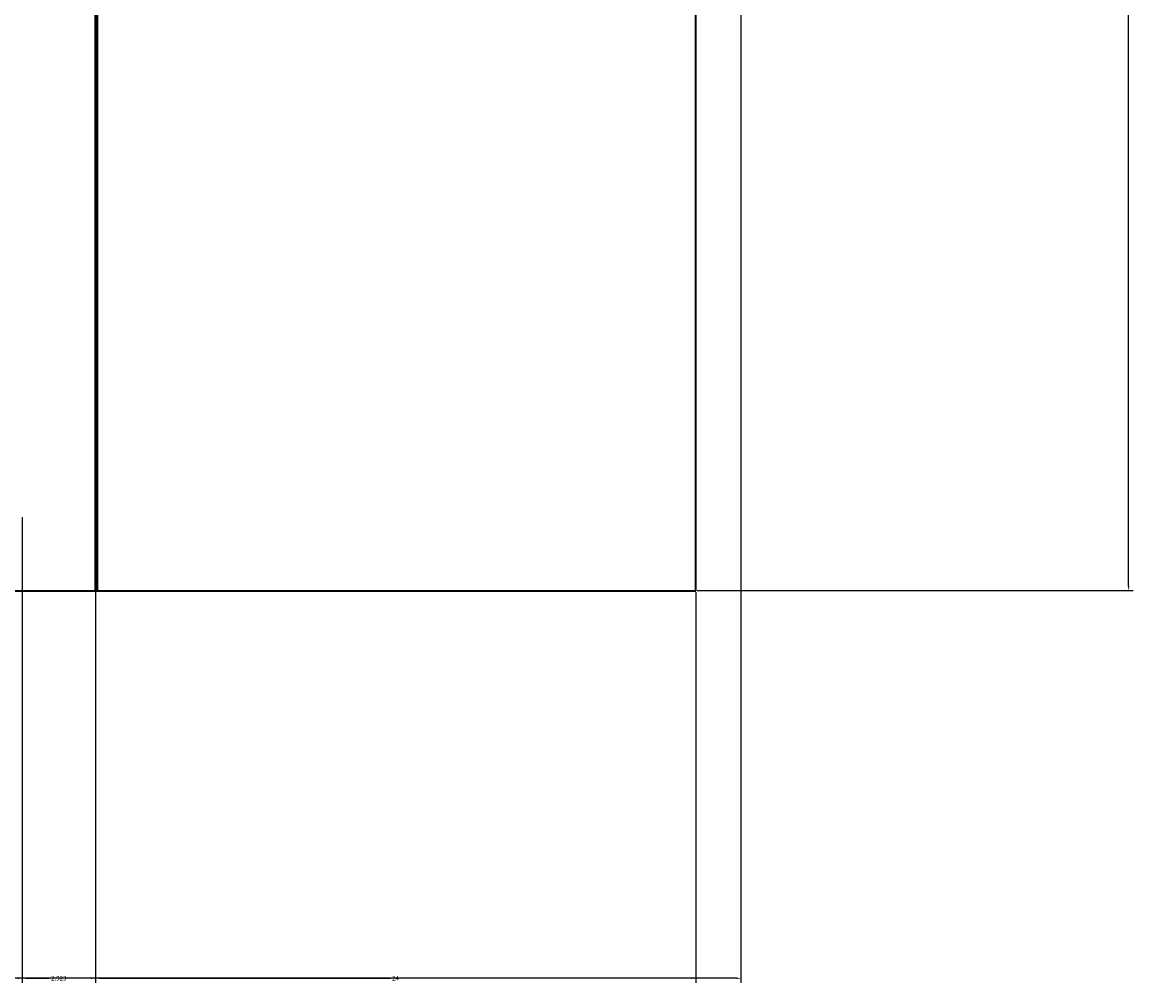
# Model space of a CAD drawing. Units: inches. Extents: x -6 to 289, y -8 to 323.
# Tile 35 of 107: x 244 to 289, y -8 to 30. Entities that reach past the tile are written whole.
import ezdxf

# ---------------------------------------------------------------- set-up
doc = ezdxf.new("R2010")
doc.units = ezdxf.units.IN
doc.header["$MEASUREMENT"] = 0
for name, color, linetype, lineweight in [('A-ANNO-DIMS', 2, 'Continuous', 18), ('A-DOOR', 3, 'Continuous', 25), ('A-ELEV', 7, 'Continuous', 35)]:
    doc.layers.add(name, color=color, linetype=linetype, lineweight=lineweight)
doc.styles.get("Standard").update_dxf_attribs({"font": 'arial.ttf'})
doc.dimstyles.get("Standard").update_dxf_attribs({"dimtxt": 0.18, "dimasz": 0.18, "dimexe": 0.18, "dimexo": 0.0625, "dimgap": 0.09, "dimtad": 0, "dimtih": 1, "dimtoh": 1, "dimdec": 4, "dimzin": 0, "dimdsep": 46, "dimtxsty": 'Standard', "dimcen": 0.09, "dimadec": 0, "dimazin": 0, "dimtfac": 1, "dimtdec": 4, "dimtofl": 0, "dimtmove": 0, "dimatfit": 3, "dimfxl": 1, "dimtolj": 1, "dimtzin": 0, "dimarcsym": 0})

# ---------------------------------------------------------------- blocks, each defined once
blk = doc.blocks.new('*D15')
at = {"layer": 'A-ANNO-DIMS', "color": 0, "lineweight": -2, "transparency": 16777216}
for p, q in [((247.164, 162.411), (247.164, 322.969)), ((247.344, 322.789), (258.944, 322.789)), ((270.984, 322.789), (259.384, 322.789)), ((271.164, 7.351), (271.164, 322.969))]:
    blk.add_line(p, q, dxfattribs=at)
at = {"layer": 'A-ANNO-DIMS', "color": 0, "transparency": 16777216}
for points in [[(247.344, 322.819), (247.344, 322.759), (247.164, 322.789)], [(270.984, 322.819), (270.984, 322.759), (271.164, 322.789)]]:
    blk.add_solid(points, dxfattribs=at)
at = {"layer": 'Defpoints', "color": 0, "transparency": 16777216}
for p in [(271.164, 322.789), (247.164, 162.348), (271.164, 7.289)]:
    blk.add_point(p, dxfattribs=at)
at = {"layer": 'A-ANNO-DIMS', "color": 0, "transparency": 16777216, "insert": (259.164, 322.789), "char_height": 0.18, "attachment_point": 5}
blk.add_mtext('\\A1;24', dxfattribs=at)
blk = doc.blocks.new('*D16')
at = {"layer": 'A-ANNO-DIMS', "color": 0, "lineweight": -2, "transparency": 16777216}
for p, q in [((9.943, 68.37), (9.943, -8.391)), ((272.973, 68.37), (272.973, -8.391)), ((10.123, -8.211), (140.993, -8.211)), ((272.793, -8.211), (141.923, -8.211))]:
    blk.add_line(p, q, dxfattribs=at)
at = {"layer": 'A-ANNO-DIMS', "color": 0, "transparency": 16777216}
for points in [[(10.123, -8.181), (10.123, -8.241), (9.943, -8.211)], [(272.793, -8.181), (272.793, -8.241), (272.973, -8.211)]]:
    blk.add_solid(points, dxfattribs=at)
at = {"layer": 'Defpoints', "color": 0, "transparency": 16777216}
for p in [(9.943, 68.432), (272.973, 68.432), (272.973, -8.211)]:
    blk.add_point(p, dxfattribs=at)
at = {"layer": 'A-ANNO-DIMS', "color": 0, "transparency": 16777216, "insert": (141.458, -8.211), "char_height": 0.18, "attachment_point": 5}
blk.add_mtext('\\A1;263.03', dxfattribs=at)
blk = doc.blocks.new('*D23')
at = {"layer": 'A-ANNO-DIMS', "color": 0, "lineweight": -2, "transparency": 16777216}
for p, q in [((259.226, 127.289), (288.653, 127.289)), ((288.473, 127.109), (288.473, 67.471)), ((288.473, 7.469), (288.473, 67.107)), ((271.226, 7.289), (288.653, 7.289))]:
    blk.add_line(p, q, dxfattribs=at)
at = {"layer": 'A-ANNO-DIMS', "color": 0, "transparency": 16777216}
for points in [[(288.443, 127.109), (288.503, 127.109), (288.473, 127.289)], [(288.443, 7.469), (288.503, 7.469), (288.473, 7.289)]]:
    blk.add_solid(points, dxfattribs=at)
at = {"layer": 'Defpoints', "color": 0, "transparency": 16777216}
for p in [(259.164, 127.289), (288.473, 127.289), (271.164, 7.289)]:
    blk.add_point(p, dxfattribs=at)
at = {"layer": 'A-ANNO-DIMS', "color": 0, "transparency": 16777216, "insert": (288.473, 67.289), "char_height": 0.18, "attachment_point": 5}
blk.add_mtext('\\A1;120', dxfattribs=at)
blk = doc.blocks.new('*D70')
at = {"layer": 'A-ANNO-DIMS', "color": 0, "lineweight": -2, "transparency": 16777216}
for p, q in [((186.36, 10.226), (186.36, -8.391)), ((244.241, 10.226), (244.241, -8.391)), ((186.54, -8.211), (214.907, -8.211)), ((244.061, -8.211), (215.694, -8.211))]:
    blk.add_line(p, q, dxfattribs=at)
at = {"layer": 'A-ANNO-DIMS', "color": 0, "transparency": 16777216}
for points in [[(186.54, -8.181), (186.54, -8.241), (186.36, -8.211)], [(244.061, -8.181), (244.061, -8.241), (244.241, -8.211)]]:
    blk.add_solid(points, dxfattribs=at)
at = {"layer": 'Defpoints', "color": 0, "transparency": 16777216}
for p in [(186.36, 10.289), (244.241, 10.289), (244.241, -8.211)]:
    blk.add_point(p, dxfattribs=at)
at = {"layer": 'A-ANNO-DIMS', "color": 0, "transparency": 16777216, "insert": (215.301, -8.211), "char_height": 0.18, "attachment_point": 5}
blk.add_mtext('\\A1;57.88', dxfattribs=at)
blk = doc.blocks.new('*D71')
at = {"layer": 'A-ANNO-DIMS', "color": 0, "lineweight": -2, "transparency": 16777216}
for p, q in [((244.241, 10.226), (244.241, -8.391)), ((247.164, 7.226), (247.164, -8.391)), ((244.421, -8.211), (245.307, -8.211)), ((246.984, -8.211), (246.098, -8.211))]:
    blk.add_line(p, q, dxfattribs=at)
at = {"layer": 'A-ANNO-DIMS', "color": 0, "transparency": 16777216}
for points in [[(244.421, -8.181), (244.421, -8.241), (244.241, -8.211)], [(246.984, -8.181), (246.984, -8.241), (247.164, -8.211)]]:
    blk.add_solid(points, dxfattribs=at)
at = {"layer": 'Defpoints', "color": 0, "transparency": 16777216}
for p in [(244.241, 10.289), (247.164, 7.289), (247.164, -8.211)]:
    blk.add_point(p, dxfattribs=at)
at = {"layer": 'A-ANNO-DIMS', "color": 0, "transparency": 16777216, "insert": (245.702, -8.211), "char_height": 0.18, "attachment_point": 5}
blk.add_mtext('\\A1;2.923', dxfattribs=at)
blk = doc.blocks.new('*D72')
at = {"layer": 'A-ANNO-DIMS', "color": 0, "lineweight": -2, "transparency": 16777216}
for p, q in [((247.164, 7.226), (247.164, -8.391)), ((271.164, 7.226), (271.164, -8.391)), ((247.344, -8.211), (258.944, -8.211)), ((270.984, -8.211), (259.384, -8.211))]:
    blk.add_line(p, q, dxfattribs=at)
at = {"layer": 'A-ANNO-DIMS', "color": 0, "transparency": 16777216}
for points in [[(247.344, -8.181), (247.344, -8.241), (247.164, -8.211)], [(270.984, -8.181), (270.984, -8.241), (271.164, -8.211)]]:
    blk.add_solid(points, dxfattribs=at)
at = {"layer": 'Defpoints', "color": 0, "transparency": 16777216}
for p in [(247.164, 7.289), (271.164, 7.289), (271.164, -8.211)]:
    blk.add_point(p, dxfattribs=at)
at = {"layer": 'A-ANNO-DIMS', "color": 0, "transparency": 16777216, "insert": (259.164, -8.211), "char_height": 0.18, "attachment_point": 5}
blk.add_mtext('\\A1;24', dxfattribs=at)

msp = doc.modelspace()

# ---------------------------------------------------------------- linework, layer by layer
at = {"layer": 'A-DOOR'}
msp.add_lwpolyline([(121.008, 51.0851), (247.2408, 51.0851), (247.2408, 7.2888), (121.008, 7.2888)], close=True, dxfattribs=at)
at = {"layer": 'A-ELEV'}
for p, q in [((247.1638, 7.2888), (247.1638, 66.2238)), ((247.2408, 66.2238), (247.2408, 7.2888)), ((271.1638, 7.2888), (271.1638, 66.2238)), ((19.1638, 7.2888), (271.1638, 7.2888)), ((247.2408, 7.2888), (271.1638, 7.2888))]:
    msp.add_line(p, q, dxfattribs=at)

# ---------------------------------------------------------------- dimensions: what is measured, and where the dimension line sits
at = {"layer": 'A-ANNO-DIMS'}
for base, p1, p2, override, picture, middle in [((271.1638, 322.7888), (247.1638, 162.3484), (271.1638, 7.2888), {"dimdec": 0, "dimlfac": 1, "dimrnd": 0, "dimzin": 0, "dimdsep": 46, "dimlunit": 2}, '*D15', (259.1638, 322.7888)), ((272.9733, -8.2112), (9.943, 68.4322), (272.9733, 68.4322), {"dimdec": 2, "dimlfac": 1, "dimrnd": 0, "dimzin": 0, "dimdsep": 46, "dimlunit": 2}, '*D16', (141.4581, -8.2112)), ((244.2408, -8.2112), (186.3604, 10.2888), (244.2408, 10.2888), {"dimdec": 2, "dimlfac": 1, "dimrnd": 0, "dimzin": 0, "dimdsep": 46, "dimlunit": 2}, '*D70', (215.3006, -8.2112)), ((247.1638, -8.2112), (244.2408, 10.2888), (247.1638, 7.2888), {"dimdec": 3, "dimlfac": 1, "dimrnd": 0, "dimzin": 0, "dimdsep": 46, "dimlunit": 2}, '*D71', (245.7023, -8.2112)), ((271.1638, -8.2112), (247.1638, 7.2888), (271.1638, 7.2888), {"dimdec": 0, "dimlfac": 1, "dimrnd": 0, "dimzin": 0, "dimdsep": 46, "dimlunit": 2}, '*D72', (259.1638, -8.2112))]:
    dim = msp.add_linear_dim(base=base, p1=p1, p2=p2, dimstyle='Standard', override=override, dxfattribs=at)
    dim.commit()
    dim.dimension.update_dxf_attribs({"geometry": picture, "text_midpoint": middle})
dim = msp.add_linear_dim(base=(288.4733, 127.2888), p1=(271.1638, 7.2888), p2=(259.1638, 127.2888), angle=90, dimstyle='Standard', override={"dimdec": 0, "dimlfac": 1, "dimrnd": 0, "dimzin": 0, "dimdsep": 46, "dimlunit": 2}, dxfattribs=at)
dim.commit()
dim.dimension.update_dxf_attribs({"geometry": '*D23', "text_midpoint": (288.4733, 67.2888)})

doc.saveas('drawing.dxf')
